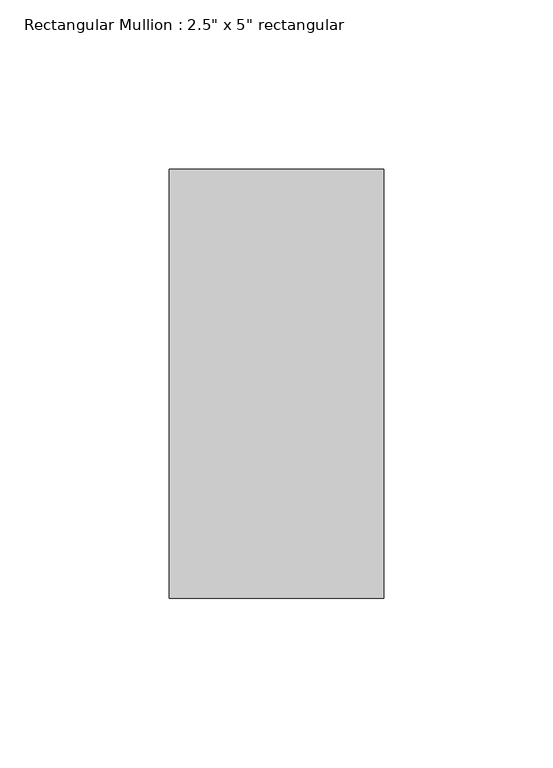
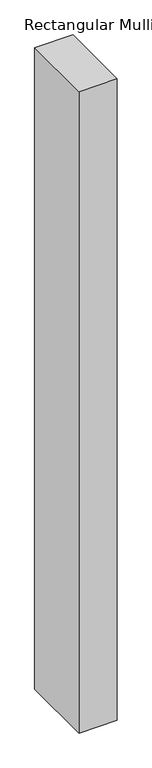
"""IFC4 building model written with IfcOpenShell, lengths in millimetres: member geometry."""

from ifc_helpers import new_model, si_unit, frame, origin, place, context, project, spatial, polyline, outline, extrude, source, transform, mapped, element, save


def member_e6b9f524(model_context):
    return source(origin(), model_context, "Body", "SweptSolid", [
        extrude(outline(polyline([(0.0, 63.5), (0.0, -63.5), (-63.5, -63.5), (-63.5, 63.5), (0.0, 63.5)])), frame((0.0, 0.0, -1123.95), z_axis=(0.0, 0.0, 1.0), x_axis=(1.0, 0.0, 0.0)), (0.0, 0.0, 1.0), 1123.95),
    ])


if __name__ == "__main__":
    model = new_model("IFC4")
    model_context = context("Model", 3, world=origin())
    ifc_project = project(units=[si_unit("LENGTHUNIT", "METRE", prefix="MILLI")], contexts=[model_context])
    site = spatial("IfcSite", under=ifc_project)
    building = spatial("IfcBuilding", under=site)
    placement = place(None, origin())
    member_shape = member_e6b9f524(model_context)
    element("IfcMember", 1, ObjectType="Rectangular Mullion : 2.5\" x 5\" rectangular", at=placement, inside=building, context=model_context, shape_type="MappedRepresentation", body=[
        mapped(member_shape, transform((0.0, 0.0, 0.0), x_axis=(1.0, 0.0, 0.0), y_axis=(0.0, 1.0, 0.0), z_axis=(0.0, 0.0, 1.0))),
    ])
    save(model, "model.ifc")

# Revit data of these elements
# Type "Rectangular Mullion : 2.5\" x 5\" rectangular"
#   built-in parameter 1007304 = 0.416667 (stored number, unit not read)
#   built-in parameter 1007301 = 0.104167 (stored number, unit not read)
#   built-in parameter 1007300 = 0.104167 (stored number, unit not read)
# Element 1 (IfcMember, "Rectangular Mullion : 2.5\" x 5\" rectangular")
#   Materials on its faces: "Door - Frame"
# Materials
#   "Door - Frame": colour RGB 118 70 51, transparency 0, Cost = 0
